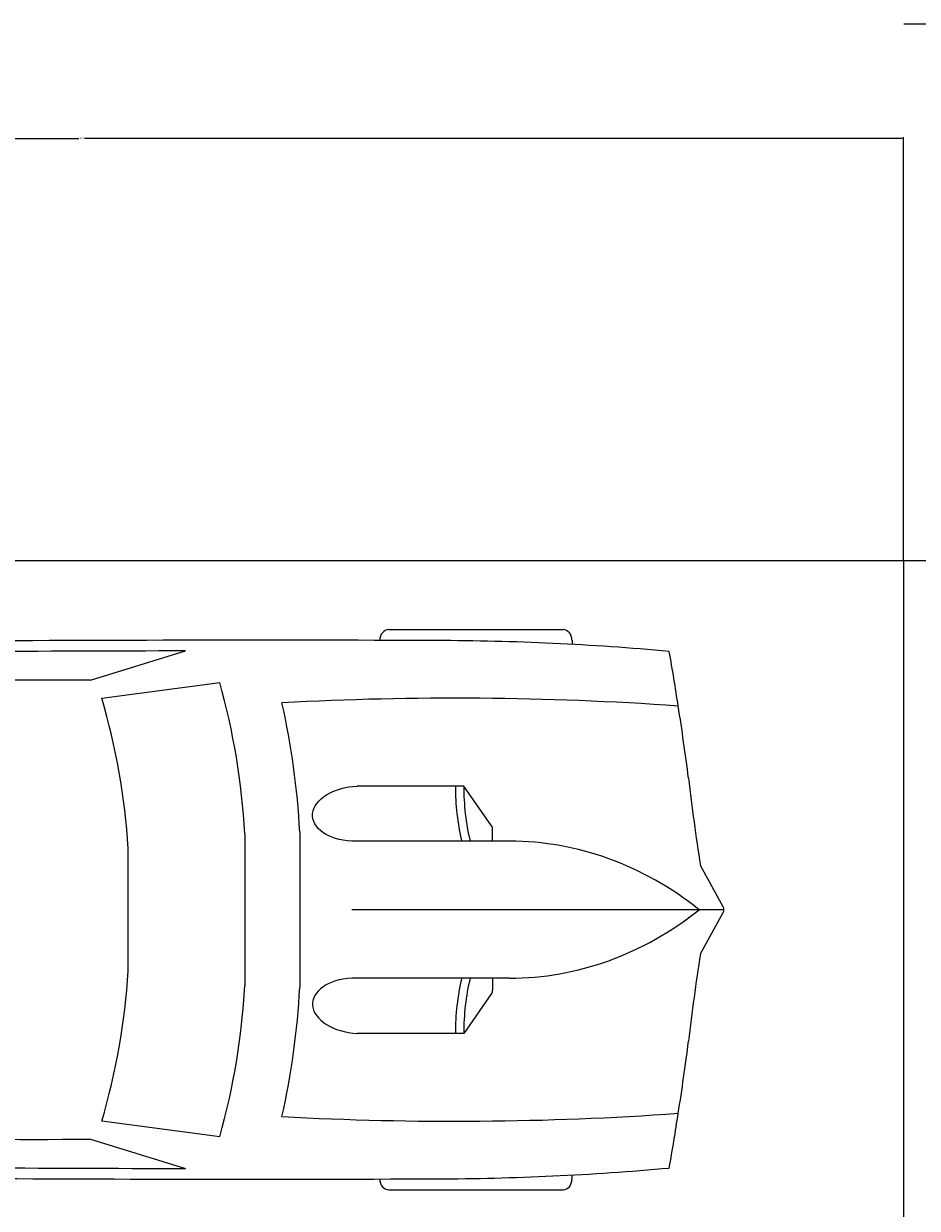
# Model space of a CAD drawing. Units: inches. Extents: x -46 to 1145, y -527 to 760.
# Tile 6 of 57: x 380 to 504, y -435 to -270. Entities that reach past the tile are written whole.
import ezdxf

# ---------------------------------------------------------------- set-up
doc = ezdxf.new("R2010")
doc.units = ezdxf.units.IN
doc.header["$MEASUREMENT"] = 0
for name, color, linetype, lineweight in [('A-ANNO-DIMS', 2, 'Continuous', 18), ('C-PKNG', 8, 'Continuous', 18), ('C-PKNG-VEHI', 8, 'Continuous', 13)]:
    doc.layers.add(name, color=color, linetype=linetype, lineweight=lineweight)
doc.styles.get("Standard").update_dxf_attribs({"font": 'arial.ttf'})
doc.dimstyles.get("Standard").update_dxf_attribs({"dimtxt": 0.18, "dimasz": 0.18, "dimexe": 0.18, "dimexo": 0.0625, "dimgap": 0.09, "dimtad": 0, "dimtih": 1, "dimtoh": 1, "dimdec": 0, "dimzin": 0, "dimdsep": 46, "dimlunit": 3, "dimtxsty": 'Standard', "dimcen": 0.09, "dimadec": 0, "dimazin": 0, "dimtfac": 1, "dimtdec": 0, "dimtofl": 0, "dimtmove": 0, "dimatfit": 3, "dimfxl": 1, "dimtolj": 1, "dimtzin": 0, "dimarcsym": 0})

# ---------------------------------------------------------------- blocks, each defined once
blk = doc.blocks.new('*U640')
for p, q in [((1182.5, 987.8), (567.7, 987.8)), ((536, 950.2), (536, 935.5)), ((1214.1, 949.7), (1214.1, 950.2)), ((2234.8, 809.5), (1898.9, 912.4)), ((1778.8, 801), (2194.7, 745.5)), ((819.6, 295.3), (917.7, 436.1)), ((917.7, 436.1), (1293.8, 436.1)), ((815.9, 241.4), (815.9, 283.3)), ((1496.5, -273.7), (1496.5, 273.7)), ((1690.4, -267.4), (1690.4, 267.4)), ((756.2, 241.4), (1312.8, 241.4)), ((2101.5, 215.8), (2101.5, -215.8)), ((83, 155.7), (2.6, 10.3)), ((0, 0), (1312.8, 0)), ((2.6, -10.3), (83, -155.7)), ((756.2, -241.4), (1312.8, -241.4)), ((815.9, -241.4), (815.9, -283.3)), ((819.6, -295.3), (917.7, -436.1)), ((917.7, -436.1), (1293.8, -436.1)), ((2194.7, -745.5), (1778.8, -801)), ((2234.8, -809.5), (1898.9, -912.4)), ((536, -950.2), (536, -935.5)), ((1214.1, -949.7), (1214.1, -950.2)), ((1182.5, -987.8), (567.7, -987.8))]:
    blk.add_line(p, q)
for centre, major_axis, ratio, start_param, end_param in [((567.7, 950.2), (0, -37.6), 0.842304, 3.141593, 4.712389), ((1182.5, 950.2), (0, 37.6), 0.842304, -1.570796, 0), ((1046.3, -12467.9), (0, 13417.1), 0.842304, 0.00281, 0.075598), ((1637.8, -268112.7), (0, 269062.9), 0.842304, -0.013397, 0.002797), ((6757.2, -699.1), (0, 7958), 0.842304, 1.367076, 1.39176), ((1637.8, -268112.7), (0, -269025.3), 0.842304, 3.133765, 3.140441), ((3436.4, 136.8), (0, 2077), 0.842304, 1.245306, 1.50788), ((2433, -93125.4), (0, -93935.2), 0.842304, 3.134049, 3.144098), ((951.8, -15086.6), (0, -15832.5), 0.842304, 3.096046, 3.200911), ((6583, -699.1), (0, -7754.7), 0.842304, 4.528606, 4.561838), ((3413.8, 136.8), (0, -2280.3), 0.842304, 4.449482, 4.652344), ((3799.7, 71.1), (0, -2021.3), 0.842304, 4.372215, 4.640744), ((-5194.2, 1330.9), (0, -6374.4), 0.842304, 1.385369, 1.434372), ((331.1, 432), (0, 696.4), 0.842304, 4.435146, 4.718221), ((360.7, 432), (0, 696.4), 0.842304, 4.435146, 4.718221), ((1290.1, 338.8), (161, -9.1), 0.603834, -1.395552, 1.581315), ((831.8, 283.3), (0, 18.8), 0.842304, 0.879714, 1.570796), ((756.2, -1185.2), (0, 1426.7), 0.842304, 0, 0.590319), ((15.8, 0), (0, -18.8), 0.842304, 4.131459, 5.293319), ((756.2, 1185.2), (0, 1426.7), 0.842304, 2.551274, 3.141593), ((-5194.2, -1330.9), (0, 6374.4), 0.842304, -1.434372, -1.385369), ((331.1, -432), (0, -696.4), 0.842304, 1.564964, 1.848039), ((360.7, -432), (0, -696.4), 0.842304, 1.564964, 1.848039), ((3799.7, -71.1), (0, -2021.3), 0.842304, -1.499151, -1.230623), ((831.8, -283.3), (0, -18.8), 0.842304, 4.712389, 5.403472), ((3413.8, -136.8), (0, -2280.3), 0.842304, -1.510751, -1.307889), ((3436.4, -136.8), (0, -2077), 0.842304, -1.50788, -1.245306), ((6583, 699.1), (0, 7754.7), 0.842304, 1.721348, 1.754579), ((6757.2, 699.1), (0, 7958), 0.842304, 1.749832, 1.774517), ((951.8, 15086.6), (0, -15832.5), 0.842304, -0.059319, 0.045547), ((2433, 93125.4), (0, -93935.2), 0.842304, -0.002505, 0.007544), ((1046.3, 12467.9), (0, -13417.1), 0.842304, -0.075598, -0.00281), ((1637.8, 268112.7), (0, -269025.3), 0.842304, 0.001152, 0.007828), ((567.7, -950.2), (0, 37.6), 0.842304, 1.570796, 3.141593), ((1637.8, 268112.7), (0, 269062.9), 0.842304, 3.138796, 3.15499), ((1182.5, -950.2), (0, -37.6), 0.842304, 0, 1.570796)]:
    blk.add_ellipse(centre, major_axis=major_axis, ratio=ratio, start_param=start_param, end_param=end_param)
at = {"extrusion": (0, 0, -1)}
blk.add_ellipse((1290.1, -338.8), major_axis=(161, 9.1), ratio=0.603834, start_param=-1.395552, end_param=1.581315, dxfattribs=at)
blk = doc.blocks.new('*D691')
at = {"layer": 'A-ANNO-DIMS', "color": 0, "lineweight": -2, "transparency": 16777216}
for p, q in [((273.52, -344.94), (273.52, -286.22)), ((273.7, -286.4), (387.23, -286.4)), ((501.55, -286.4), (388.02, -286.4)), ((501.73, -344.94), (501.73, -286.22))]:
    blk.add_line(p, q, dxfattribs=at)
at = {"layer": 'A-ANNO-DIMS', "color": 0, "transparency": 16777216}
for points in [[(273.7, -286.37), (273.7, -286.43), (273.52, -286.4)], [(501.55, -286.37), (501.55, -286.43), (501.73, -286.4)]]:
    blk.add_solid(points, dxfattribs=at)
at = {"layer": 'Defpoints', "color": 0, "transparency": 16777216}
for p in [(501.73, -286.4), (273.52, -345), (501.73, -345)]:
    blk.add_point(p, dxfattribs=at)
at = {"layer": 'A-ANNO-DIMS', "color": 0, "transparency": 16777216, "insert": (387.62, -286.4), "char_height": 0.18, "attachment_point": 5}
blk.add_mtext('\\A1;228.2', dxfattribs=at)
blk = doc.blocks.new('*D700')
at = {"layer": 'A-ANNO-DIMS', "color": 0, "lineweight": -2, "transparency": 16777216}
for p, q in [((501.79, -270.48), (560.51, -270.48)), ((560.33, -270.66), (560.33, -307.56)), ((560.33, -344.82), (560.33, -307.92)), ((501.79, -345), (560.51, -345))]:
    blk.add_line(p, q, dxfattribs=at)
at = {"layer": 'A-ANNO-DIMS', "color": 0, "transparency": 16777216}
for points in [[(560.3, -270.66), (560.36, -270.66), (560.33, -270.48)], [(560.3, -344.82), (560.36, -344.82), (560.33, -345)]]:
    blk.add_solid(points, dxfattribs=at)
at = {"layer": 'Defpoints', "color": 0, "transparency": 16777216}
for p in [(501.73, -270.48), (501.73, -345), (560.33, -345)]:
    blk.add_point(p, dxfattribs=at)
at = {"layer": 'A-ANNO-DIMS', "color": 0, "transparency": 16777216, "insert": (560.33, -307.74), "char_height": 0.18, "attachment_point": 5}
blk.add_mtext('\\A1;74.52', dxfattribs=at)
blk = doc.blocks.new('*D702')
at = {"layer": 'A-ANNO-DIMS', "color": 0, "lineweight": -2, "transparency": 16777216}
for p, q in [((189.63, -39.48), (1145.34, -39.48)), ((1145.16, -39.66), (1145.16, -249.3)), ((1145.16, -459.3), (1145.16, -249.66)), ((183.63, -459.48), (1145.34, -459.48))]:
    blk.add_line(p, q, dxfattribs=at)
at = {"layer": 'A-ANNO-DIMS', "color": 0, "transparency": 16777216}
for points in [[(1145.13, -39.66), (1145.19, -39.66), (1145.16, -39.48)], [(1145.13, -459.3), (1145.19, -459.3), (1145.16, -459.48)]]:
    blk.add_solid(points, dxfattribs=at)
at = {"layer": 'Defpoints', "color": 0, "transparency": 16777216}
for p in [(189.56, -39.48), (1145.16, -39.48), (183.56, -459.48)]:
    blk.add_point(p, dxfattribs=at)
at = {"layer": 'A-ANNO-DIMS', "color": 0, "transparency": 16777216, "insert": (1145.16, -249.48), "char_height": 0.18, "attachment_point": 5}
blk.add_mtext('\\A1;420', dxfattribs=at)

msp = doc.modelspace()

# ---------------------------------------------------------------- linework, layer by layer
at = {"layer": 'C-PKNG'}
msp.add_lwpolyline([(501.7297, -443.2988), (273.5156, -443.2988), (273.5156, -345.0009), (501.7297, -345.0009)], close=True, dxfattribs=at)

# ---------------------------------------------------------------- block references
at = {"layer": 'C-PKNG-VEHI', "xscale": 0.0393700787401575, "yscale": 0.0393700787401575, "zscale": 0.0393700787401575, "rotation": 180}
msp.add_blockref('*U640', (476.808, -393.4831), dxfattribs=at)

# ---------------------------------------------------------------- dimensions: what is measured, and where the dimension line sits
at = {"layer": 'A-ANNO-DIMS'}
for base, p1, p2, angle, override, picture, middle in [((1145.1637, -39.4824), (183.5637, -459.4824), (189.5637, -39.4824), 90, {"dimdec": 0, "dimlfac": 1, "dimrnd": 0, "dimzin": 0, "dimdsep": 46, "dimlunit": 2}, '*D702', (1145.1637, -249.4824)), ((560.3297, -345.0009), (501.7297, -270.4792), (501.7297, -345.0009), 270, {"dimdec": 2, "dimlfac": 1, "dimrnd": 0, "dimzin": 0, "dimdsep": 46, "dimlunit": 2}, '*D700', (560.3297, -307.74))]:
    dim = msp.add_linear_dim(base=base, p1=p1, p2=p2, angle=angle, dimstyle='Standard', override=override, dxfattribs=at)
    dim.commit()
    dim.dimension.update_dxf_attribs({"geometry": picture, "text_midpoint": middle})
dim = msp.add_linear_dim(base=(501.7297, -286.4009), p1=(273.5156, -345.0009), p2=(501.7297, -345.0009), dimstyle='Standard', override={"dimdec": 1, "dimlfac": 1, "dimrnd": 0, "dimzin": 0, "dimdsep": 46, "dimlunit": 2}, dxfattribs=at)
dim.commit()
dim.dimension.update_dxf_attribs({"geometry": '*D691', "text_midpoint": (387.6227, -286.4009)})

doc.saveas('drawing.dxf')
